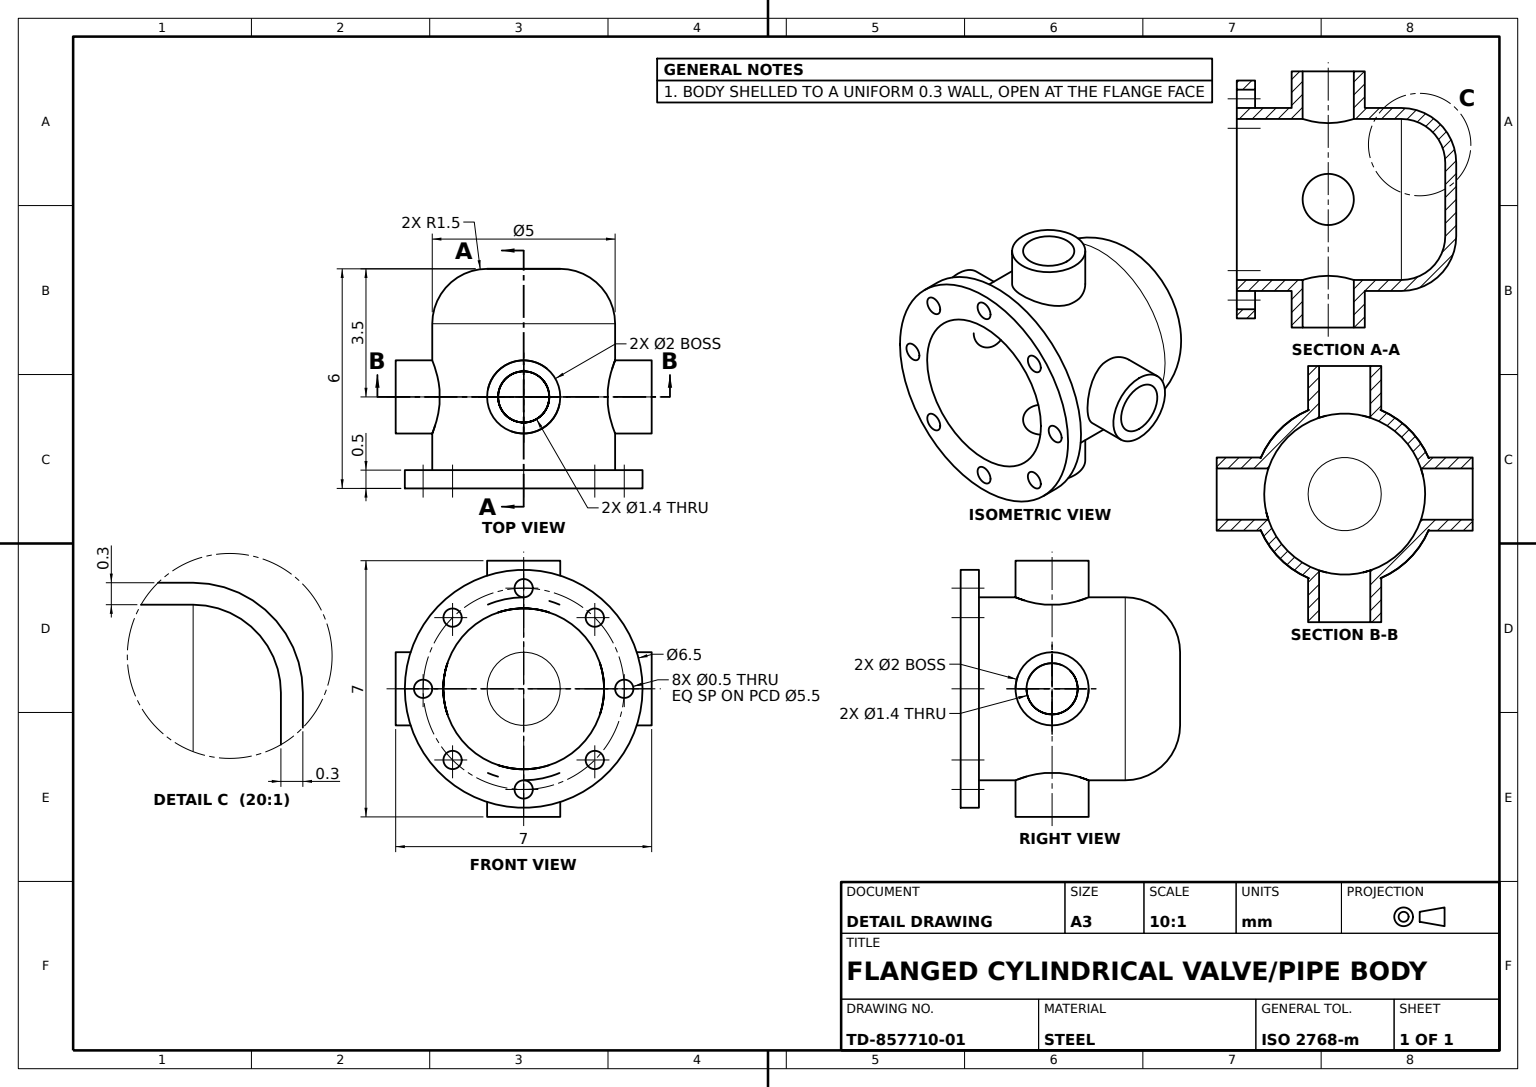
SolidWorks part; units mm, degrees
material "Plain Carbon Steel"
ref_plane "Front Plane" through (0, 0, 0) normal (0, 0, 1) x (1, 0, 0)
ref_plane "Top Plane" through (0, 0, 0) normal (0, 1, 0) x (1, 0, 0)
ref_plane "Right Plane" through (0, 0, 0) normal (1, 0, 0) x (0, 0, -1)
sketch "Body Profile Sketch" plane through (0, 0, 0) normal (0, 0, 1) x (1, 0, 0)
  line L0 (0, 0) -> (0, 5.5)
  line L1 (0, 5.5) -> (-2.5, 5.5)
  line L2 (-2.5, 5.5) -> (-2.5, 1.5)
  line L3 (0, 0) -> (-1, 0)
  arc A0 (-2.5, 1.5) -> (-1, 0) centre (-1, 1.5) ccw
  dimension "D1" = 5.5
  dimension "D2" = 1
  dimension "D3" = 2.5
revolve "Body Revolve" add sketch "Body Profile Sketch" angle 360 about L0
shell "Body Shell 0.3" thickness 0.3
sketch "Flange Sketch Ø6.5" plane through (0, 5.5, 0) normal (0, 1, 0) x (1, 0, 0)
  circle A0 centre (0, 0) radius 3.25
  dimension "D1" = 6.5
extrude "Flange" add sketch "Flange Sketch Ø6.5" along normal blind 0.5
sketch "Flange Bore Sketch" plane through (0, 6, 0) normal (0, 1, 0) x (1, 0, 0)
  circle A1 centre (0, 0) radius 2.2 construction
  circle A2 centre (0, 0) radius 2.2
extrude "Flange Bore" cut sketch "Flange Bore Sketch" against normal blind 0.5
sketch "Flange Bolt Holes Sketch" plane through (0, 6, 0) normal (0, 1, 0) x (1, 0, 0)
  circle A1 centre (0, 2.75) radius 0.25
  circle A2 centre (1.9445, 1.9445) radius 0.25
  circle A3 centre (2.75, 0) radius 0.25
  circle A4 centre (1.9445, -1.9445) radius 0.25
  circle A5 centre (0, -2.75) radius 0.25
  circle A6 centre (-1.9445, -1.9445) radius 0.25
  circle A7 centre (-2.75, 0) radius 0.25
  circle A8 centre (-1.9445, 1.9445) radius 0.25
  dimension "D1" = 2.75
  dimension "D2" = 0.5
  dimension "D4" = 1.9445
  dimension "D5" = 1.9445
  dimension "D6" = 0.8055
  dimension "D3" = 8
extrude "Flange Bolt Holes 8x" cut sketch "Flange Bolt Holes Sketch" against normal blind 0.5
ref_plane "Plane1" through (0, 0, 3.5) normal (0, 0, 1) x (1, 0, 0)
sketch "Side Port Boss Sketch Ø2" plane through (0, 0, 3.5) normal (0, 0, 1) x (1, 0, 0)
  circle A0 centre (0, 3.5) radius 1
  dimension "D1" = 2
  dimension "D2" = 3.25
  dimension "D3" = 3.5
extrude "Side Port Boss" add sketch "Side Port Boss Sketch Ø2" against normal blind 1.2
sketch "Side Port Bore Sketch Ø1.4" plane through (0, 0, 3.5) normal (0, 0, 1) x (1, 0, 0)
  circle A0 centre (0, 3.5) radius 0.7
  dimension "D1" = 1.4
extrude "Side Port Bore Ø1.4" cut sketch "Side Port Bore Sketch Ø1.4" against normal blind 1.5
pattern_circular "Side Port Pattern 4x" count 4 over 360 about axis through (0, 0, 0) along (0, 1, 0) of "Side Port Boss", "Side Port Bore Ø1.4"
